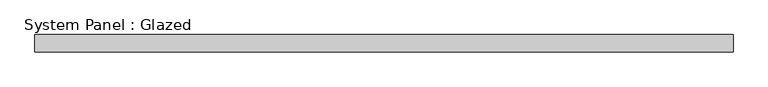
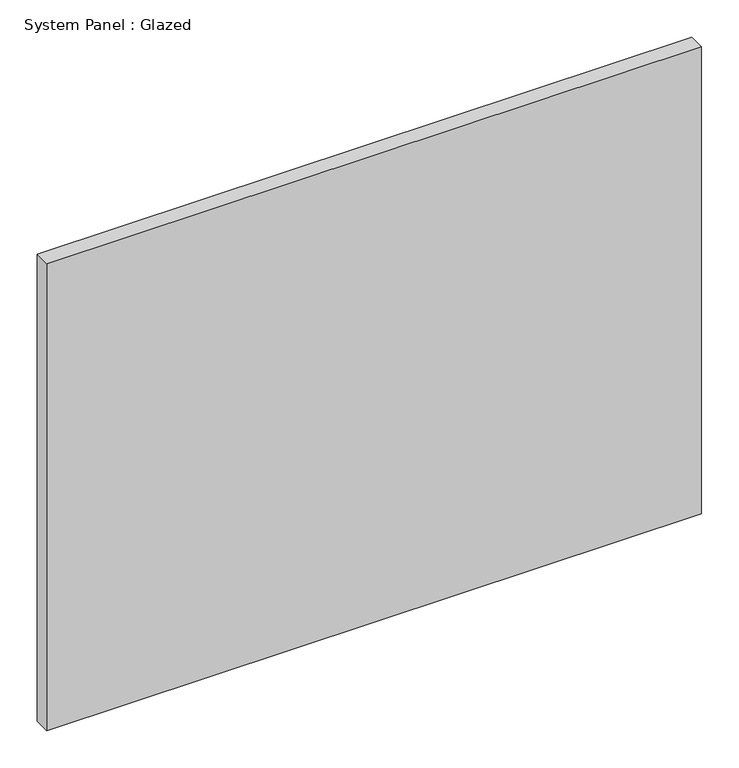
"""IFC4 building model written with IfcOpenShell, lengths in millimetres: plate geometry, System Panel : Glazed."""

from ifc_helpers import new_model, si_unit, origin, origin_with_axes, place, context, project, spatial, polyline, outline, extrude, source, transform, mapped, element, save


def system_panel_glazed_cb69acbc(model_context):
    return source(origin(), model_context, "Body", "SweptSolid", [
        extrude(outline(polyline([(508.92075, 19.05), (-508.92075, 19.05), (-508.92075, 44.45), (508.92075, 44.45), (508.92075, 19.05)])), origin_with_axes(), (0.0, 0.0, 1.0), 767.461),
    ])


if __name__ == "__main__":
    model = new_model("IFC4")
    model_context = context("Model", 3, world=origin())
    ifc_project = project(units=[si_unit("LENGTHUNIT", "METRE", prefix="MILLI")], contexts=[model_context])
    site = spatial("IfcSite", under=ifc_project)
    building = spatial("IfcBuilding", under=site)
    placement = place(None, origin())
    system_panel_glazed_shape = system_panel_glazed_cb69acbc(model_context)
    element("IfcPlate", 1, ObjectType="System Panel : Glazed", at=placement, inside=building, context=model_context, shape_type="MappedRepresentation", body=[
        mapped(system_panel_glazed_shape, transform((0.0, 0.0, 0.0), x_axis=(1.0, 0.0, 0.0), y_axis=(0.0, 1.0, 0.0), z_axis=(0.0, 0.0, 1.0))),
    ])
    save(model, "model.ifc")

# Revit data of these elements
# Type "System Panel : Glazed"
#   Construction Type Id = "GSP4R"
#   Analytic Construction = "1/8 in Pilkington single glazing"
#   Visual Light Transmittance = 0.9
#   Solar Heat Gain Coefficient = 0.86
#   Heat Transfer Coefficient (U) = 1.18115 BTU/(h·ft²·°F)
#   Define Thermal Properties by = 1
# Element 1 (IfcPlate, "System Panel : Glazed")
#   Materials on its faces: "Glass"
# Materials
#   "Glass": class "Glass", colour RGB 0 128 192, transparency 0.75, Description = "Soda Lime Glass", Cost = 0
